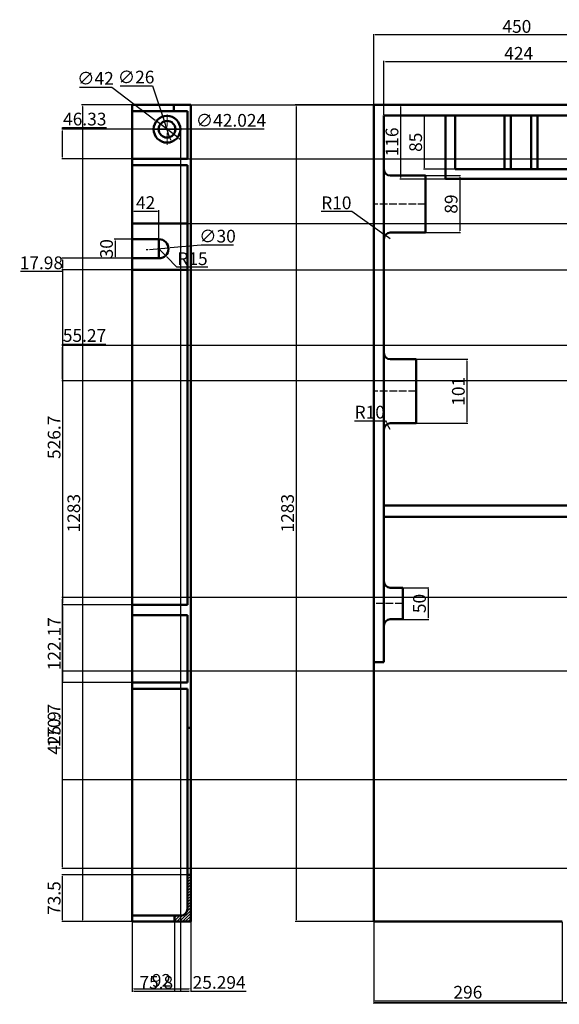
# Model space of a CAD drawing. Units: millimetres. Extents: x 1408 to 3734, y 1022 to 2569.
# Tile 1 of 3: x 1408 to 2256, y 1022 to 2569. Entities that reach past the tile are written whole.
import ezdxf

# ---------------------------------------------------------------- set-up
doc = ezdxf.new("R2010")
doc.units = ezdxf.units.MM
doc.linetypes.add('ACAD_ISO02W100', pattern=[15, 12, -3])
doc.linetypes.add('CENTER2', pattern=[28.575, 19.05, -3.175, 3.175, -3.175])
for name, color, linetype, lineweight in [('M-CNTR', 1, 'CENTER2', 18), ('M-DIMS', 2, 'Continuous', 25), ('M-HATC', 8, 'Continuous', 18), ('M-HIDN', 4, 'ACAD_ISO02W100', 25), ('M-OUTL', 7, 'Continuous', 50)]:
    doc.layers.add(name, color=color, linetype=linetype, lineweight=lineweight)
doc.styles.get("Standard").update_dxf_attribs({"font": 'arial.ttf'})
doc.dimstyles.new('ISO-25', dxfattribs={"dimtxt": 20, "dimasz": 2.5, "dimexe": 1.25, "dimexo": 0.625, "dimtad": 1, "dimtoh": 1, "dimdec": 0, "dimtxsty": 'Standard', "dimcen": 2.5, "dimadec": 0, "dimazin": 0, "dimtfac": 1, "dimtdec": 0, "dimtmove": 0, "dimatfit": 3, "dimfxl": 1, "dimarcsym": 0})

# ---------------------------------------------------------------- blocks, each defined once
blk = doc.blocks.new('*U3')
at = {"layer": 'M-CNTR', "color": 0, "transparency": 16777216}
for p, q in [((0, 4.2), (0, 24.5)), ((-24.5, 0), (-4.2, 0)), ((4.2, 0), (24.5, 0)), ((0, -24.5), (0, -4.2))]:
    blk.add_line(p, q, dxfattribs=at)
at = {"layer": 'M-CNTR', "color": 0, "linetype": 'Continuous', "transparency": 16777216}
for p, q in [((-2.1, 0), (2.1, 0)), ((0, -2.1), (0, 2.1))]:
    blk.add_line(p, q, dxfattribs=at)
blk = doc.blocks.new('*D4')
at = {"layer": 'Defpoints', "color": 0, "transparency": 16777216}
for p in [(1585, 2435.4), (1506.7, 1152.1), (1585, 1152.1)]:
    blk.add_point(p, dxfattribs=at)
at = {"layer": 'M-DIMS', "color": 0, "lineweight": -2, "transparency": 16777216}
for p, q in [((1584.3, 2435.4), (1505.4, 2435.4)), ((1506.7, 2432.9), (1506.7, 1154.6)), ((1584.3, 1152.1), (1505.4, 1152.1))]:
    blk.add_line(p, q, dxfattribs=at)
at = {"layer": 'M-DIMS', "color": 0, "transparency": 16777216}
for points in [[(1506.2, 2432.9), (1507.1, 2432.9), (1506.7, 2435.4)], [(1506.2, 1154.6), (1507.1, 1154.6), (1506.7, 1152.1)]]:
    blk.add_solid(points, dxfattribs=at)
at = {"layer": 'M-DIMS', "color": 0, "transparency": 16777216, "insert": (1495.8, 1793.7), "char_height": 20, "attachment_point": 5, "rotation": 90}
blk.add_mtext('1283', dxfattribs=at)
blk = doc.blocks.new('*D5')
at = {"layer": 'Defpoints', "color": 0, "transparency": 16777216}
for p in [(1585, 1152.1), (1677, 1152.1), (1677, 1046.1)]:
    blk.add_point(p, dxfattribs=at)
at = {"layer": 'M-DIMS', "color": 0, "lineweight": -2, "transparency": 16777216}
for p, q in [((1585, 1151.5), (1585, 1044.9)), ((1677, 1151.5), (1677, 1044.9)), ((1587.5, 1046.1), (1674.5, 1046.1))]:
    blk.add_line(p, q, dxfattribs=at)
at = {"layer": 'M-DIMS', "color": 0, "transparency": 16777216}
for points in [[(1587.5, 1046.5), (1587.5, 1045.7), (1585, 1046.1)], [(1674.5, 1046.5), (1674.5, 1045.7), (1677, 1046.1)]]:
    blk.add_solid(points, dxfattribs=at)
at = {"layer": 'M-DIMS', "color": 0, "transparency": 16777216, "insert": (1631, 1056.9), "char_height": 20, "attachment_point": 5}
blk.add_mtext('92', dxfattribs=at)
blk = doc.blocks.new('*D6')
at = {"layer": 'Defpoints', "color": 0, "transparency": 16777216}
for p in [(1964.7, 1152.1), (2260.7, 1152.1), (2260.7, 1027.5)]:
    blk.add_point(p, dxfattribs=at)
at = {"layer": 'M-DIMS', "color": 0, "lineweight": -2, "transparency": 16777216}
for p, q in [((1964.7, 1151.5), (1964.7, 1026.2)), ((2260.7, 1151.5), (2260.7, 1026.2)), ((1967.2, 1027.5), (2258.2, 1027.5))]:
    blk.add_line(p, q, dxfattribs=at)
at = {"layer": 'M-DIMS', "color": 0, "transparency": 16777216}
for points in [[(1967.2, 1027.9), (1967.2, 1027.1), (1964.7, 1027.5)], [(2258.2, 1027.9), (2258.2, 1027.1), (2260.7, 1027.5)]]:
    blk.add_solid(points, dxfattribs=at)
at = {"layer": 'M-DIMS', "color": 0, "transparency": 16777216, "insert": (2112.7, 1038.3), "char_height": 20, "attachment_point": 5}
blk.add_mtext('296', dxfattribs=at)
blk = doc.blocks.new('*D7')
at = {"layer": 'Defpoints', "color": 0, "transparency": 16777216}
for p in [(2814.7, 1219.4), (1964.7, 1152.1), (2814.7, 1025)]:
    blk.add_point(p, dxfattribs=at)
at = {"layer": 'M-DIMS', "color": 0, "lineweight": -2, "transparency": 16777216}
for p, q in [((2814.7, 1218.8), (2814.7, 1023.8)), ((1964.7, 1151.5), (1964.7, 1023.8)), ((1967.2, 1025), (2812.2, 1025))]:
    blk.add_line(p, q, dxfattribs=at)
at = {"layer": 'M-DIMS', "color": 0, "transparency": 16777216}
for points in [[(1967.2, 1025.5), (1967.2, 1024.6), (1964.7, 1025)], [(2812.2, 1025.5), (2812.2, 1024.6), (2814.7, 1025)]]:
    blk.add_solid(points, dxfattribs=at)
at = {"layer": 'M-DIMS', "color": 0, "transparency": 16777216, "insert": (2389.7, 1035.9), "char_height": 20, "attachment_point": 5}
blk.add_mtext('850', dxfattribs=at)
blk = doc.blocks.new('*D8')
at = {"layer": 'Defpoints', "color": 0, "transparency": 16777216}
for p in [(3556.7, 1373.9), (1964.7, 1152.1), (3556.7, 1024.2)]:
    blk.add_point(p, dxfattribs=at)
at = {"layer": 'M-DIMS', "color": 0, "lineweight": -2, "transparency": 16777216}
for p, q in [((3556.7, 1373.3), (3556.7, 1022.9)), ((1964.7, 1151.5), (1964.7, 1022.9)), ((1967.2, 1024.2), (3554.2, 1024.2))]:
    blk.add_line(p, q, dxfattribs=at)
at = {"layer": 'M-DIMS', "color": 0, "transparency": 16777216}
for points in [[(1967.2, 1024.6), (1967.2, 1023.8), (1964.7, 1024.2)], [(3554.2, 1024.6), (3554.2, 1023.8), (3556.7, 1024.2)]]:
    blk.add_solid(points, dxfattribs=at)
at = {"layer": 'M-DIMS', "color": 0, "transparency": 16777216, "insert": (2760.7, 1035), "char_height": 20, "attachment_point": 5}
blk.add_mtext('1592', dxfattribs=at)
blk = doc.blocks.new('*D9')
at = {"layer": 'Defpoints', "color": 0, "transparency": 16777216}
for p in [(1964.7, 2435.4), (1842.6, 1152.1), (1964.7, 1152.1)]:
    blk.add_point(p, dxfattribs=at)
at = {"layer": 'M-DIMS', "color": 0, "lineweight": -2, "transparency": 16777216}
for p, q in [((1964.1, 2435.4), (1841.4, 2435.4)), ((1842.6, 2432.9), (1842.6, 1154.6)), ((1964.1, 1152.1), (1841.4, 1152.1))]:
    blk.add_line(p, q, dxfattribs=at)
at = {"layer": 'M-DIMS', "color": 0, "transparency": 16777216}
for points in [[(1842.2, 2432.9), (1843, 2432.9), (1842.6, 2435.4)], [(1842.2, 1154.6), (1843, 1154.6), (1842.6, 1152.1)]]:
    blk.add_solid(points, dxfattribs=at)
at = {"layer": 'M-DIMS', "color": 0, "transparency": 16777216, "insert": (1831.8, 1793.7), "char_height": 20, "attachment_point": 5, "rotation": 90}
blk.add_mtext('1283', dxfattribs=at)
blk = doc.blocks.new('*D13')
at = {"layer": 'Defpoints', "color": 0, "transparency": 16777216}
for p in [(1964.7, 2545.3), (1964.7, 2435.4), (2414.7, 2435.4)]:
    blk.add_point(p, dxfattribs=at)
at = {"layer": 'M-DIMS', "color": 0, "lineweight": -2, "transparency": 16777216}
for p, q in [((1964.7, 2436), (1964.7, 2546.6)), ((2412.2, 2545.3), (1967.2, 2545.3)), ((2414.7, 2436), (2414.7, 2546.6))]:
    blk.add_line(p, q, dxfattribs=at)
at = {"layer": 'M-DIMS', "color": 0, "transparency": 16777216}
for points in [[(1967.2, 2545.7), (1967.2, 2544.9), (1964.7, 2545.3)], [(2412.2, 2545.7), (2412.2, 2544.9), (2414.7, 2545.3)]]:
    blk.add_solid(points, dxfattribs=at)
at = {"layer": 'M-DIMS', "color": 0, "transparency": 16777216, "insert": (2189.7, 2556.1), "char_height": 20, "attachment_point": 5}
blk.add_mtext('450', dxfattribs=at)
blk = doc.blocks.new('*D20')
at = {"layer": 'Defpoints', "color": 0, "transparency": 16777216}
for p in [(1623, 2409.8), (1656.5, 2384.4)]:
    blk.add_point(p, dxfattribs=at)
at = {"layer": 'M-DIMS', "color": 0, "lineweight": -2, "transparency": 16777216}
for p, q in [((1502.2, 2463.1), (1553, 2463.1)), ((1553, 2463.1), (1621, 2411.3)), ((1656.5, 2384.4), (1623, 2409.8)), ((1658.5, 2382.9), (1660.5, 2381.4))]:
    blk.add_line(p, q, dxfattribs=at)
at = {"layer": 'M-DIMS', "color": 0, "transparency": 16777216}
for points in [[(1621.3, 2411.7), (1620.8, 2411), (1623, 2409.8)], [(1658.7, 2383.2), (1658.2, 2382.6), (1656.5, 2384.4)]]:
    blk.add_solid(points, dxfattribs=at)
at = {"layer": 'M-DIMS', "color": 0, "transparency": 16777216, "insert": (1527.3, 2474.5), "char_height": 20, "attachment_point": 5}
blk.add_mtext('∅42', dxfattribs=at)
blk = doc.blocks.new('*D21')
at = {"layer": 'Defpoints', "color": 0, "transparency": 16777216}
for p in [(1635.6, 2409.5), (1643.9, 2384.7)]:
    blk.add_point(p, dxfattribs=at)
at = {"layer": 'M-DIMS', "color": 0, "lineweight": -2, "transparency": 16777216}
for p, q in [((1566, 2465.1), (1617, 2465.1)), ((1617, 2465.1), (1634.8, 2411.9)), ((1643.9, 2384.7), (1635.6, 2409.5)), ((1644.7, 2382.3), (1645.5, 2379.9))]:
    blk.add_line(p, q, dxfattribs=at)
at = {"layer": 'M-DIMS', "color": 0, "transparency": 16777216}
for points in [[(1635.2, 2412), (1634.4, 2411.8), (1635.6, 2409.5)], [(1645.1, 2382.4), (1644.3, 2382.2), (1643.9, 2384.7)]]:
    blk.add_solid(points, dxfattribs=at)
at = {"layer": 'M-DIMS', "color": 0, "transparency": 16777216, "insert": (1591.2, 2476.5), "char_height": 20, "attachment_point": 5}
blk.add_mtext('∅26', dxfattribs=at)
blk = doc.blocks.new('*D22')
at = {"layer": 'Defpoints', "color": 0, "transparency": 16777216}
for p in [(1612.2, 2208), (1642.1, 2210.6)]:
    blk.add_point(p, dxfattribs=at)
at = {"layer": 'M-DIMS', "color": 0, "lineweight": -2, "transparency": 16777216}
for p, q in [((1693.4, 2215.1), (1644.6, 2210.8)), ((1744.3, 2215.1), (1693.4, 2215.1)), ((1609.7, 2207.7), (1607.2, 2207.5)), ((1612.2, 2208), (1642.1, 2210.6))]:
    blk.add_line(p, q, dxfattribs=at)
at = {"layer": 'M-DIMS', "color": 0, "transparency": 16777216}
for points in [[(1609.7, 2208.1), (1609.7, 2207.3), (1612.2, 2208)], [(1644.5, 2211.2), (1644.6, 2210.4), (1642.1, 2210.6)]]:
    blk.add_solid(points, dxfattribs=at)
at = {"layer": 'M-DIMS', "color": 0, "transparency": 16777216, "insert": (1719.1, 2226.5), "char_height": 20, "attachment_point": 5}
blk.add_mtext('∅30', dxfattribs=at)
blk = doc.blocks.new('*D23')
at = {"layer": 'Defpoints', "color": 0, "transparency": 16777216}
for p in [(1627.1, 2268.5), (1585, 2224.3), (1627.1, 2224.3)]:
    blk.add_point(p, dxfattribs=at)
at = {"layer": 'M-DIMS', "color": 0, "lineweight": -2, "transparency": 16777216}
for p, q in [((1585, 2224.9), (1585, 2269.8)), ((1587.5, 2268.5), (1624.6, 2268.5)), ((1627.1, 2224.9), (1627.1, 2269.8))]:
    blk.add_line(p, q, dxfattribs=at)
at = {"layer": 'M-DIMS', "color": 0, "transparency": 16777216}
for points in [[(1587.5, 2268.9), (1587.5, 2268.1), (1585, 2268.5)], [(1624.6, 2268.9), (1624.6, 2268.1), (1627.1, 2268.5)]]:
    blk.add_solid(points, dxfattribs=at)
at = {"layer": 'M-DIMS', "color": 0, "transparency": 16777216, "insert": (1606.1, 2279.2), "char_height": 20, "attachment_point": 5}
blk.add_mtext('42', dxfattribs=at)
blk = doc.blocks.new('*D24')
at = {"layer": 'Defpoints', "color": 0, "transparency": 16777216}
for p in [(1585, 2224.3), (1558.1, 2194.3), (1585, 2194.3)]:
    blk.add_point(p, dxfattribs=at)
at = {"layer": 'M-DIMS', "color": 0, "lineweight": -2, "transparency": 16777216}
for p, q in [((1584.3, 2224.3), (1556.9, 2224.3)), ((1558.1, 2221.8), (1558.1, 2196.8)), ((1584.3, 2194.3), (1556.9, 2194.3))]:
    blk.add_line(p, q, dxfattribs=at)
at = {"layer": 'M-DIMS', "color": 0, "transparency": 16777216}
for points in [[(1557.7, 2221.8), (1558.6, 2221.8), (1558.1, 2224.3)], [(1557.7, 2196.8), (1558.6, 2196.8), (1558.1, 2194.3)]]:
    blk.add_solid(points, dxfattribs=at)
at = {"layer": 'M-DIMS', "color": 0, "transparency": 16777216, "insert": (1547.3, 2209.3), "char_height": 20, "attachment_point": 5, "rotation": 90}
blk.add_mtext('30', dxfattribs=at)
blk = doc.blocks.new('*D30')
at = {"layer": 'Defpoints', "color": 0, "transparency": 16777216}
for p in [(2031.3, 2035.6), (2031.3, 1935), (2111.2, 1935)]:
    blk.add_point(p, dxfattribs=at)
at = {"layer": 'M-DIMS', "color": 0, "lineweight": -2, "transparency": 16777216}
for p, q in [((2031.9, 2035.6), (2112.4, 2035.6)), ((2111.2, 2033.1), (2111.2, 1937.5)), ((2031.9, 1935), (2112.4, 1935))]:
    blk.add_line(p, q, dxfattribs=at)
at = {"layer": 'M-DIMS', "color": 0, "transparency": 16777216}
for points in [[(2110.8, 2033.1), (2111.6, 2033.1), (2111.2, 2035.6)], [(2110.8, 1937.5), (2111.6, 1937.5), (2111.2, 1935)]]:
    blk.add_solid(points, dxfattribs=at)
at = {"layer": 'M-DIMS', "color": 0, "transparency": 16777216, "insert": (2100.3, 1985.3), "char_height": 20, "attachment_point": 5, "rotation": 90}
blk.add_mtext('101', dxfattribs=at)
blk = doc.blocks.new('*D31')
at = {"layer": 'Defpoints', "color": 0, "transparency": 16777216}
for p in [(2010.5, 1676.6), (2010.5, 1626.9), (2050.1, 1626.9)]:
    blk.add_point(p, dxfattribs=at)
at = {"layer": 'M-DIMS', "color": 0, "lineweight": -2, "transparency": 16777216}
for p, q in [((2011.1, 1676.6), (2051.3, 1676.6)), ((2050.1, 1674.1), (2050.1, 1629.4)), ((2011.1, 1626.9), (2051.3, 1626.9))]:
    blk.add_line(p, q, dxfattribs=at)
at = {"layer": 'M-DIMS', "color": 0, "transparency": 16777216}
for points in [[(2049.6, 1674.1), (2050.5, 1674.1), (2050.1, 1676.6)], [(2049.6, 1629.4), (2050.5, 1629.4), (2050.1, 1626.9)]]:
    blk.add_solid(points, dxfattribs=at)
at = {"layer": 'M-DIMS', "color": 0, "transparency": 16777216, "insert": (2039.2, 1651.8), "char_height": 20, "attachment_point": 5, "rotation": 90}
blk.add_mtext('50', dxfattribs=at)
blk = doc.blocks.new('*D32')
at = {"layer": 'Defpoints', "color": 0, "transparency": 16777216}
for p in [(2046.2, 2324.2), (2046.2, 2234.8), (2099.8, 2234.8)]:
    blk.add_point(p, dxfattribs=at)
at = {"layer": 'M-DIMS', "color": 0, "lineweight": -2, "transparency": 16777216}
for p, q in [((2046.8, 2324.2), (2101.1, 2324.2)), ((2099.8, 2321.7), (2099.8, 2237.3)), ((2046.8, 2234.8), (2101.1, 2234.8))]:
    blk.add_line(p, q, dxfattribs=at)
at = {"layer": 'M-DIMS', "color": 0, "transparency": 16777216}
for points in [[(2099.4, 2321.7), (2100.2, 2321.7), (2099.8, 2324.2)], [(2099.4, 2237.3), (2100.2, 2237.3), (2099.8, 2234.8)]]:
    blk.add_solid(points, dxfattribs=at)
at = {"layer": 'M-DIMS', "color": 0, "transparency": 16777216, "insert": (2089, 2279.5), "char_height": 20, "attachment_point": 5, "rotation": 90}
blk.add_mtext('89', dxfattribs=at)
blk = doc.blocks.new('*D33')
at = {"layer": 'Defpoints', "color": 0, "transparency": 16777216}
for p in [(1982.5, 2230.7), (1990.7, 2224.8)]:
    blk.add_point(p, dxfattribs=at)
at = {"layer": 'M-DIMS', "color": 0, "lineweight": -2, "transparency": 16777216}
for p, q in [((1882, 2268.1), (1930.4, 2268.1)), ((1930.4, 2268.1), (1980.5, 2232.1)), ((1990.7, 2224.8), (1982.5, 2230.7))]:
    blk.add_line(p, q, dxfattribs=at)
at = {"layer": 'M-DIMS', "color": 0, "transparency": 16777216}
blk.add_solid([(1980.7, 2232.4), (1980.3, 2231.8), (1982.5, 2230.7)], dxfattribs=at)
at = {"layer": 'M-DIMS', "color": 0, "transparency": 16777216, "insert": (1905.9, 2278.9), "char_height": 20, "attachment_point": 5}
blk.add_mtext('R10', dxfattribs=at)
blk = doc.blocks.new('*D34')
at = {"layer": 'Defpoints', "color": 0, "transparency": 16777216}
for p in [(1980.7, 2503.2), (1980.7, 2418.9), (2404.5, 2417.1)]:
    blk.add_point(p, dxfattribs=at)
at = {"layer": 'M-DIMS', "color": 0, "lineweight": -2, "transparency": 16777216}
for p, q in [((1980.7, 2419.6), (1980.7, 2504.4)), ((2402, 2503.2), (1983.2, 2503.2)), ((2404.5, 2417.7), (2404.5, 2504.4))]:
    blk.add_line(p, q, dxfattribs=at)
at = {"layer": 'M-DIMS', "color": 0, "transparency": 16777216}
for points in [[(1983.2, 2503.6), (1983.2, 2502.8), (1980.7, 2503.2)], [(2402, 2503.6), (2402, 2502.8), (2404.5, 2503.2)]]:
    blk.add_solid(points, dxfattribs=at)
at = {"layer": 'M-DIMS', "color": 0, "transparency": 16777216, "insert": (2192.6, 2513.8), "char_height": 20, "attachment_point": 5}
blk.add_mtext('424', dxfattribs=at)
blk = doc.blocks.new('*D35')
at = {"layer": 'Defpoints', "color": 0, "transparency": 16777216}
for p in [(2190.9, 2418.9), (2044, 2334.2), (2252.1, 2334.2)]:
    blk.add_point(p, dxfattribs=at)
at = {"layer": 'M-DIMS', "color": 0, "lineweight": -2, "transparency": 16777216}
for p, q in [((2190.3, 2418.9), (2042.8, 2418.9)), ((2044, 2416.4), (2044, 2336.7)), ((2251.5, 2334.2), (2042.8, 2334.2))]:
    blk.add_line(p, q, dxfattribs=at)
at = {"layer": 'M-DIMS', "color": 0, "transparency": 16777216}
for points in [[(2043.6, 2416.4), (2044.4, 2416.4), (2044, 2418.9)], [(2043.6, 2336.7), (2044.4, 2336.7), (2044, 2334.2)]]:
    blk.add_solid(points, dxfattribs=at)
at = {"layer": 'M-DIMS', "color": 0, "transparency": 16777216, "insert": (2033.2, 2376.6), "char_height": 20, "attachment_point": 5, "rotation": 90}
blk.add_mtext('85', dxfattribs=at)
blk = doc.blocks.new('*D36')
at = {"layer": 'Defpoints', "color": 0, "transparency": 16777216}
for p in [(2189.7, 2435.4), (2006.9, 2318.9), (2231.1, 2318.9)]:
    blk.add_point(p, dxfattribs=at)
at = {"layer": 'M-DIMS', "color": 0, "lineweight": -2, "transparency": 16777216}
for p, q in [((2189.1, 2435.4), (2005.6, 2435.4)), ((2006.9, 2432.9), (2006.9, 2321.4)), ((2230.5, 2318.9), (2005.6, 2318.9))]:
    blk.add_line(p, q, dxfattribs=at)
at = {"layer": 'M-DIMS', "color": 0, "transparency": 16777216}
for points in [[(2006.5, 2432.9), (2007.3, 2432.9), (2006.9, 2435.4)], [(2006.5, 2321.4), (2007.3, 2321.4), (2006.9, 2318.9)]]:
    blk.add_solid(points, dxfattribs=at)
at = {"layer": 'M-DIMS', "color": 0, "transparency": 16777216, "insert": (1996, 2377.2), "char_height": 20, "attachment_point": 5, "rotation": 90}
blk.add_mtext('116', dxfattribs=at)
blk = doc.blocks.new('*D40')
at = {"layer": 'Defpoints', "color": 0, "transparency": 16777216}
for p in [(1660.8, 2397.1), (1585, 2350.8), (1660.8, 1042.8)]:
    blk.add_point(p, dxfattribs=at)
at = {"layer": 'M-DIMS', "color": 0, "lineweight": -2, "transparency": 16777216}
for p, q in [((1660.8, 2396.5), (1660.8, 1041.6)), ((1585, 2350.2), (1585, 1041.6)), ((1587.5, 1042.8), (1658.3, 1042.8))]:
    blk.add_line(p, q, dxfattribs=at)
at = {"layer": 'M-DIMS', "color": 0, "transparency": 16777216}
for points in [[(1587.5, 1043.3), (1587.5, 1042.4), (1585, 1042.8)], [(1658.3, 1043.3), (1658.3, 1042.4), (1660.8, 1042.8)]]:
    blk.add_solid(points, dxfattribs=at)
at = {"layer": 'M-DIMS', "color": 0, "transparency": 16777216, "insert": (1622.9, 1053.7), "char_height": 20, "attachment_point": 5}
blk.add_mtext('75.8', dxfattribs=at)
blk = doc.blocks.new('*D41')
at = {"layer": 'Defpoints', "color": 0, "transparency": 16777216}
for p in [(1475.7, 2397.1), (1660.8, 2397.1), (1585, 2350.8)]:
    blk.add_point(p, dxfattribs=at)
at = {"layer": 'M-DIMS', "color": 0, "lineweight": -2, "transparency": 16777216}
for p, q in [((1475.7, 2397.1), (1475.7, 2399.6)), ((1475.7, 2399.6), (1544.6, 2399.6)), ((1660.1, 2397.1), (1474.5, 2397.1)), ((1475.7, 2353.3), (1475.7, 2394.6)), ((1584.3, 2350.8), (1474.5, 2350.8))]:
    blk.add_line(p, q, dxfattribs=at)
at = {"layer": 'M-DIMS', "color": 0, "transparency": 16777216}
for points in [[(1475.3, 2394.6), (1476.1, 2394.6), (1475.7, 2397.1)], [(1475.3, 2353.3), (1476.1, 2353.3), (1475.7, 2350.8)]]:
    blk.add_solid(points, dxfattribs=at)
at = {"layer": 'M-DIMS', "color": 0, "transparency": 16777216, "insert": (1510.5, 2410.5), "char_height": 20, "attachment_point": 5}
blk.add_mtext('46.33', dxfattribs=at)
blk = doc.blocks.new('*D42')
at = {"layer": 'Defpoints', "color": 0, "transparency": 16777216}
for p in [(1677, 2435.4), (1671.8, 2350.8), (3665.9, 2350.8)]:
    blk.add_point(p, dxfattribs=at)
at = {"layer": 'M-DIMS', "color": 0, "lineweight": -2, "transparency": 16777216}
for p, q in [((1677.6, 2435.4), (3667.2, 2435.4)), ((3665.9, 2432.9), (3665.9, 2353.3)), ((1672.5, 2350.8), (3667.2, 2350.8))]:
    blk.add_line(p, q, dxfattribs=at)
at = {"layer": 'M-DIMS', "color": 0, "transparency": 16777216}
for points in [[(3665.5, 2432.9), (3666.4, 2432.9), (3665.9, 2435.4)], [(3665.5, 2353.3), (3666.4, 2353.3), (3665.9, 2350.8)]]:
    blk.add_solid(points, dxfattribs=at)
at = {"layer": 'M-DIMS', "color": 0, "transparency": 16777216, "insert": (3655.1, 2393.1), "char_height": 20, "attachment_point": 5, "rotation": 90}
blk.add_mtext('84.6', dxfattribs=at)
blk = doc.blocks.new('*D43')
at = {"layer": 'Defpoints', "color": 0, "transparency": 16777216}
for p in [(1671.8, 2350.8), (1671.8, 2249.2), (3665.9, 2249.2)]:
    blk.add_point(p, dxfattribs=at)
at = {"layer": 'M-DIMS', "color": 0, "lineweight": -2, "transparency": 16777216}
for p, q in [((1672.5, 2350.8), (3667.2, 2350.8)), ((3665.9, 2348.3), (3665.9, 2251.7)), ((1672.5, 2249.2), (3667.2, 2249.2))]:
    blk.add_line(p, q, dxfattribs=at)
at = {"layer": 'M-DIMS', "color": 0, "transparency": 16777216}
for points in [[(3665.5, 2348.3), (3666.4, 2348.3), (3665.9, 2350.8)], [(3665.5, 2251.7), (3666.4, 2251.7), (3665.9, 2249.2)]]:
    blk.add_solid(points, dxfattribs=at)
at = {"layer": 'M-DIMS', "color": 0, "transparency": 16777216, "insert": (3655.1, 2300), "char_height": 20, "attachment_point": 5, "rotation": 90}
blk.add_mtext('101.6', dxfattribs=at)
blk = doc.blocks.new('*D44')
at = {"layer": 'Defpoints', "color": 0, "transparency": 16777216}
for p in [(1671.8, 2249.2), (1671.8, 2176.3), (3665.9, 2176.3)]:
    blk.add_point(p, dxfattribs=at)
at = {"layer": 'M-DIMS', "color": 0, "lineweight": -2, "transparency": 16777216}
for p, q in [((1672.5, 2249.2), (3667.2, 2249.2)), ((3665.9, 2246.7), (3665.9, 2178.8)), ((1672.5, 2176.3), (3667.2, 2176.3))]:
    blk.add_line(p, q, dxfattribs=at)
at = {"layer": 'M-DIMS', "color": 0, "transparency": 16777216}
for points in [[(3665.5, 2246.7), (3666.4, 2246.7), (3665.9, 2249.2)], [(3665.5, 2178.8), (3666.4, 2178.8), (3665.9, 2176.3)]]:
    blk.add_solid(points, dxfattribs=at)
at = {"layer": 'M-DIMS', "color": 0, "transparency": 16777216, "insert": (3655.1, 2212.7), "char_height": 20, "attachment_point": 5, "rotation": 90}
blk.add_mtext('72.9', dxfattribs=at)
blk = doc.blocks.new('*D45')
at = {"layer": 'Defpoints', "color": 0, "transparency": 16777216}
for p in [(1671.8, 2176.3), (1475.7, 1649.6), (1671.8, 1649.6)]:
    blk.add_point(p, dxfattribs=at)
at = {"layer": 'M-DIMS', "color": 0, "lineweight": -2, "transparency": 16777216}
for p, q in [((1671.2, 2176.3), (1474.5, 2176.3)), ((1475.7, 2173.8), (1475.7, 1652.1)), ((1671.2, 1649.6), (1474.5, 1649.6))]:
    blk.add_line(p, q, dxfattribs=at)
at = {"layer": 'M-DIMS', "color": 0, "transparency": 16777216}
for points in [[(1475.3, 2173.8), (1476.1, 2173.8), (1475.7, 2176.3)], [(1475.3, 1652.1), (1476.1, 1652.1), (1475.7, 1649.6)]]:
    blk.add_solid(points, dxfattribs=at)
at = {"layer": 'M-DIMS', "color": 0, "transparency": 16777216, "insert": (1464.9, 1912.9), "char_height": 20, "attachment_point": 5, "rotation": 90}
blk.add_mtext('526.7', dxfattribs=at)
blk = doc.blocks.new('*D46')
at = {"layer": 'Defpoints', "color": 0, "transparency": 16777216}
for p in [(1671.8, 1649.6), (1475.7, 1527.4), (1671.8, 1527.4)]:
    blk.add_point(p, dxfattribs=at)
at = {"layer": 'M-DIMS', "color": 0, "lineweight": -2, "transparency": 16777216}
for p, q in [((1671.2, 1649.6), (1474.5, 1649.6)), ((1475.7, 1647.1), (1475.7, 1529.9)), ((1671.2, 1527.4), (1474.5, 1527.4))]:
    blk.add_line(p, q, dxfattribs=at)
at = {"layer": 'M-DIMS', "color": 0, "transparency": 16777216}
for points in [[(1475.3, 1647.1), (1476.1, 1647.1), (1475.7, 1649.6)], [(1475.3, 1529.9), (1476.1, 1529.9), (1475.7, 1527.4)]]:
    blk.add_solid(points, dxfattribs=at)
at = {"layer": 'M-DIMS', "color": 0, "transparency": 16777216, "insert": (1465, 1588.5), "char_height": 20, "attachment_point": 5, "rotation": 90}
blk.add_mtext('122.17', dxfattribs=at)
blk = doc.blocks.new('*D47')
at = {"layer": 'Defpoints', "color": 0, "transparency": 16777216}
for p in [(1585, 2194.3), (1475.7, 2176.3), (1585, 2176.3)]:
    blk.add_point(p, dxfattribs=at)
at = {"layer": 'M-DIMS', "color": 0, "lineweight": -2, "transparency": 16777216}
for p, q in [((1584.3, 2194.3), (1474.5, 2194.3)), ((1475.7, 2191.8), (1475.7, 2178.8)), ((1475.7, 2173.8), (1409.4, 2173.8)), ((1584.3, 2176.3), (1474.5, 2176.3)), ((1475.7, 2176.3), (1475.7, 2173.8))]:
    blk.add_line(p, q, dxfattribs=at)
at = {"layer": 'M-DIMS', "color": 0, "transparency": 16777216}
for points in [[(1475.3, 2191.8), (1476.1, 2191.8), (1475.7, 2194.3)], [(1475.3, 2178.8), (1476.1, 2178.8), (1475.7, 2176.3)]]:
    blk.add_solid(points, dxfattribs=at)
at = {"layer": 'M-DIMS', "color": 0, "transparency": 16777216, "insert": (1442.3, 2184.6), "char_height": 20, "attachment_point": 5}
blk.add_mtext('17.98', dxfattribs=at)
blk = doc.blocks.new('*D48')
at = {"layer": 'Defpoints', "color": 0, "transparency": 16777216}
for p in [(1475.7, 1225.6), (1677, 1225.6), (1677, 1152.1)]:
    blk.add_point(p, dxfattribs=at)
at = {"layer": 'M-DIMS', "color": 0, "lineweight": -2, "transparency": 16777216}
for p, q in [((1676.3, 1225.6), (1474.5, 1225.6)), ((1475.7, 1154.6), (1475.7, 1223.1)), ((1676.3, 1152.1), (1474.5, 1152.1))]:
    blk.add_line(p, q, dxfattribs=at)
at = {"layer": 'M-DIMS', "color": 0, "transparency": 16777216}
for points in [[(1475.3, 1223.1), (1476.1, 1223.1), (1475.7, 1225.6)], [(1475.3, 1154.6), (1476.1, 1154.6), (1475.7, 1152.1)]]:
    blk.add_solid(points, dxfattribs=at)
at = {"layer": 'M-DIMS', "color": 0, "transparency": 16777216, "insert": (1464.9, 1188.8), "char_height": 20, "attachment_point": 5, "rotation": 90}
blk.add_mtext('73.5', dxfattribs=at)
blk = doc.blocks.new('*D49')
at = {"layer": 'Defpoints', "color": 0, "transparency": 16777216}
for p in [(1651.7, 1152.1), (1677, 1152.1), (1677, 1042.8)]:
    blk.add_point(p, dxfattribs=at)
at = {"layer": 'M-DIMS', "color": 0, "lineweight": -2, "transparency": 16777216}
for p, q in [((1651.7, 1151.5), (1651.7, 1041.6)), ((1677, 1151.5), (1677, 1041.6)), ((1654.2, 1042.8), (1674.5, 1042.8)), ((1677, 1042.8), (1764, 1042.8))]:
    blk.add_line(p, q, dxfattribs=at)
at = {"layer": 'M-DIMS', "color": 0, "transparency": 16777216}
for points in [[(1654.2, 1043.3), (1654.2, 1042.4), (1651.7, 1042.8)], [(1674.5, 1043.3), (1674.5, 1042.4), (1677, 1042.8)]]:
    blk.add_solid(points, dxfattribs=at)
at = {"layer": 'M-DIMS', "color": 0, "transparency": 16777216, "insert": (1721.7, 1053.7), "char_height": 20, "attachment_point": 5}
blk.add_mtext('25.294', dxfattribs=at)
blk = doc.blocks.new('*D50')
at = {"layer": 'Defpoints', "color": 0, "transparency": 16777216}
for p in [(1475.7, 2057.1), (3047.3, 2057.1), (3014.5, 2001.8)]:
    blk.add_point(p, dxfattribs=at)
at = {"layer": 'M-DIMS', "color": 0, "lineweight": -2, "transparency": 16777216}
for p, q in [((1475.7, 2057.1), (1475.7, 2059.6)), ((1475.7, 2059.6), (1543.8, 2059.6)), ((3046.6, 2057.1), (1474.5, 2057.1)), ((1475.7, 2004.3), (1475.7, 2054.6)), ((3013.9, 2001.8), (1474.5, 2001.8))]:
    blk.add_line(p, q, dxfattribs=at)
at = {"layer": 'M-DIMS', "color": 0, "transparency": 16777216}
for points in [[(1475.3, 2054.6), (1476.1, 2054.6), (1475.7, 2057.1)], [(1475.3, 2004.3), (1476.1, 2004.3), (1475.7, 2001.8)]]:
    blk.add_solid(points, dxfattribs=at)
at = {"layer": 'M-DIMS', "color": 0, "transparency": 16777216, "insert": (1510.1, 2070.4), "char_height": 20, "attachment_point": 5}
blk.add_mtext('55.27', dxfattribs=at)
blk = doc.blocks.new('*D60')
at = {"layer": 'Defpoints', "color": 0, "transparency": 16777216}
for p in [(1475.7, 1661.3), (2298.6, 1661.3), (2298.6, 1235.4)]:
    blk.add_point(p, dxfattribs=at)
at = {"layer": 'M-DIMS', "color": 0, "lineweight": -2, "transparency": 16777216}
for p, q in [((2298, 1661.3), (1474.5, 1661.3)), ((1475.7, 1237.9), (1475.7, 1658.8)), ((2298, 1235.4), (1474.5, 1235.4))]:
    blk.add_line(p, q, dxfattribs=at)
at = {"layer": 'M-DIMS', "color": 0, "transparency": 16777216}
for points in [[(1475.3, 1658.8), (1476.1, 1658.8), (1475.7, 1661.3)], [(1475.3, 1237.9), (1476.1, 1237.9), (1475.7, 1235.4)]]:
    blk.add_solid(points, dxfattribs=at)
at = {"layer": 'M-DIMS', "color": 0, "transparency": 16777216, "insert": (1464.9, 1448.3), "char_height": 20, "attachment_point": 5, "rotation": 90}
blk.add_mtext('425.9', dxfattribs=at)
blk = doc.blocks.new('*D62')
at = {"layer": 'Defpoints', "color": 0, "transparency": 16777216}
for p in [(1475.7, 1545.3), (2452.5, 1545.3), (2379.1, 1374.6)]:
    blk.add_point(p, dxfattribs=at)
at = {"layer": 'M-DIMS', "color": 0, "lineweight": -2, "transparency": 16777216}
for p, q in [((2451.8, 1545.3), (1474.5, 1545.3)), ((1475.7, 1377.1), (1475.7, 1542.8)), ((2378.5, 1374.6), (1474.5, 1374.6))]:
    blk.add_line(p, q, dxfattribs=at)
at = {"layer": 'M-DIMS', "color": 0, "transparency": 16777216}
for points in [[(1475.3, 1542.8), (1476.1, 1542.8), (1475.7, 1545.3)], [(1475.3, 1377.1), (1476.1, 1377.1), (1475.7, 1374.6)]]:
    blk.add_solid(points, dxfattribs=at)
at = {"layer": 'M-DIMS', "color": 0, "transparency": 16777216, "insert": (1464.9, 1459.9), "char_height": 20, "attachment_point": 5, "rotation": 90}
blk.add_mtext('170.7', dxfattribs=at)
blk = doc.blocks.new('*D85')
at = {"layer": 'Defpoints', "color": 0, "transparency": 16777216}
for p in [(1618.7, 2397.1), (1660.8, 2397.1)]:
    blk.add_point(p, dxfattribs=at)
at = {"layer": 'M-DIMS', "color": 0, "lineweight": -2, "transparency": 16777216}
for p, q in [((1616.2, 2397.1), (1613.7, 2397.1)), ((1618.7, 2397.1), (1660.8, 2397.1)), ((1687.3, 2397.1), (1663.3, 2397.1)), ((1792.6, 2397.1), (1687.3, 2397.1))]:
    blk.add_line(p, q, dxfattribs=at)
at = {"layer": 'M-DIMS', "color": 0, "transparency": 16777216}
for points in [[(1616.2, 2397.5), (1616.2, 2396.7), (1618.7, 2397.1)], [(1663.3, 2397.5), (1663.3, 2396.7), (1660.8, 2397.1)]]:
    blk.add_solid(points, dxfattribs=at)
at = {"layer": 'M-DIMS', "color": 0, "transparency": 16777216, "insert": (1740.3, 2408.5), "char_height": 20, "attachment_point": 5}
blk.add_mtext('∅42.024', dxfattribs=at)
blk = doc.blocks.new('*D86')
at = {"layer": 'Defpoints', "color": 0, "transparency": 16777216}
for p in [(1627.1, 2209.3), (1637.5, 2198.5)]:
    blk.add_point(p, dxfattribs=at)
at = {"layer": 'M-DIMS', "color": 0, "lineweight": -2, "transparency": 16777216}
for p, q in [((1627.1, 2209.3), (1637.5, 2198.5)), ((1655.2, 2180.1), (1639.3, 2196.7)), ((1703.7, 2180.1), (1655.2, 2180.1))]:
    blk.add_line(p, q, dxfattribs=at)
at = {"layer": 'M-DIMS', "color": 0, "transparency": 16777216}
blk.add_solid([(1639.6, 2196.9), (1639, 2196.4), (1637.5, 2198.5)], dxfattribs=at)
at = {"layer": 'M-DIMS', "color": 0, "transparency": 16777216, "insert": (1679.8, 2191), "char_height": 20, "attachment_point": 5}
blk.add_mtext('R15', dxfattribs=at)
blk = doc.blocks.new('*D87')
at = {"layer": 'Defpoints', "color": 0, "transparency": 16777216}
for p in [(1985.8, 1933.8), (1990.7, 1925)]:
    blk.add_point(p, dxfattribs=at)
at = {"layer": 'M-DIMS', "color": 0, "lineweight": -2, "transparency": 16777216}
for p, q in [((1934.6, 1939.1), (1983, 1939.1)), ((1983, 1939.1), (1984.6, 1936)), ((1990.7, 1925), (1985.8, 1933.8))]:
    blk.add_line(p, q, dxfattribs=at)
at = {"layer": 'M-DIMS', "color": 0, "transparency": 16777216}
blk.add_solid([(1985, 1936.2), (1984.3, 1935.8), (1985.8, 1933.8)], dxfattribs=at)
at = {"layer": 'M-DIMS', "color": 0, "transparency": 16777216, "insert": (1958.5, 1949.9), "char_height": 20, "attachment_point": 5}
blk.add_mtext('R10', dxfattribs=at)

msp = doc.modelspace()

# ---------------------------------------------------------------- hatches: boundary and pattern name
at = {"layer": 'M-HATC'}
h = msp.add_hatch(dxfattribs=at)
h.set_pattern_fill('ANSI31', color=256)
h.paths.add_polyline_path([(1676.9655, 1219.3757), (1676.9655, 1225.5822), (1671.843, 1225.5822), (1671.843, 1219.3757), (1671.843, 1171.4252, -0.414213562), (1661.843, 1161.4252), (1651.6714, 1161.4252), (1651.6714, 1152.0867), (1676.9655, 1152.0867)])

# ---------------------------------------------------------------- linework, layer by layer
at = {"layer": 'M-HIDN'}
for p, q in [((2046.202, 2279.513), (1964.6991, 2279.513)), ((2031.2921, 1985.3002), (1964.6991, 1985.3002)), ((2010.4639, 1651.7582), (1964.6991, 1651.7582))]:
    msp.add_line(p, q, dxfattribs=at)
at = {"layer": 'M-OUTL'}
for p, q in [((1676.9655, 2435.3757), (1584.9655, 2435.3757)), ((1584.9655, 2435.3757), (1584.9655, 1152.0867)), ((1650.3694, 2425.5407), (1650.3694, 2435.3757)), ((1676.9655, 2435.3757), (1676.9655, 1219.3757)), ((1964.6991, 2435.3757), (1964.6991, 1219.3757)), ((1964.6991, 2435.3757), (2414.6991, 2435.3757)), ((1671.843, 2425.5407), (1584.9655, 2425.5407)), ((1671.843, 2425.5407), (1671.843, 2350.7788)), ((1980.6517, 2418.9311), (2401.1247, 2418.9311)), ((1980.6517, 2418.9311), (1980.6517, 2334.2036)), ((2077.4791, 2418.9311), (2077.4791, 2318.9311)), ((2092.8085, 2418.9311), (2092.8085, 2334.2032)), ((2170.0319, 2418.9311), (2170.0319, 2334.2032)), ((2180.0319, 2334.2032), (2180.0319, 2418.9311)), ((2212.0319, 2418.9311), (2212.0319, 2334.2032)), ((2222.0319, 2334.2032), (2222.0319, 2418.9311)), ((1584.9655, 2350.7788), (1671.843, 2350.7788)), ((1671.843, 2340.7788), (1584.9655, 2340.7788)), ((1671.843, 2340.7788), (1671.843, 1649.6019)), ((1980.6517, 2224.8225), (1980.6517, 2334.2036)), ((2046.202, 2324.2036), (1990.6517, 2324.2036)), ((2046.202, 2234.8225), (2046.202, 2324.2036)), ((2092.8085, 2334.2032), (2411.4791, 2334.2032)), ((2077.4791, 2318.9311), (2384.7504, 2318.9311)), ((1584.9655, 2249.1777), (1671.843, 2249.1777)), ((1990.6517, 2234.8225), (2046.202, 2234.8225)), ((1584.9655, 2224.2646), (1627.1403, 2224.2646)), ((1627.1403, 2224.2646), (1627.1403, 2194.2646)), ((1980.6517, 2224.8225), (1980.6517, 2045.5771)), ((1627.1403, 2194.2646), (1584.9655, 2194.2646)), ((1671.843, 2176.2838), (1584.9655, 2176.2838)), ((1980.6517, 1973.3926), (1980.6517, 2045.5771)), ((2031.2921, 2035.5771), (1990.6517, 2035.5771)), ((2031.2921, 1935.0233), (2031.2921, 2035.5771)), ((1980.6517, 1925.0233), (1980.6517, 1973.3926)), ((1990.6517, 1935.0233), (2031.2921, 1935.0233)), ((1980.6517, 1925.0233), (1980.6517, 1686.6065)), ((1980.6517, 1805.8149), (2798.6154, 1805.8149)), ((1980.6517, 1787.9634), (2798.6154, 1787.9634)), ((1980.6517, 1616.9099), (1980.6517, 1686.6065)), ((2010.4639, 1676.6065), (1990.6517, 1676.6065)), ((2010.4639, 1626.9099), (2010.4639, 1676.6065)), ((1584.9655, 1649.6019), (1671.843, 1649.6019)), ((1671.843, 1633.6019), (1584.9655, 1633.6019)), ((1671.843, 1633.6019), (1671.843, 1527.4292)), ((1990.6517, 1626.9099), (2010.4639, 1626.9099)), ((1980.6517, 1616.9099), (1980.6517, 1559.5606)), ((1964.6991, 1559.5606), (1980.6517, 1559.5606)), ((1584.9655, 1527.4292), (1671.843, 1527.4292)), ((1671.843, 1517.4292), (1584.9655, 1517.4292)), ((1671.843, 1517.4292), (1671.843, 1219.3757)), ((1671.843, 1456.2631), (1676.9655, 1456.2631)), ((1671.843, 1225.5822), (1676.9655, 1225.5822)), ((1671.843, 1219.3757), (1671.843, 1171.4252)), ((1676.9655, 1219.3757), (1676.9655, 1152.0867)), ((1964.6991, 1219.3757), (1964.6991, 1152.0867)), ((1661.843, 1161.4252), (1584.9655, 1161.4252)), ((1651.6714, 1161.4252), (1651.6714, 1152.0867)), ((1676.9655, 1152.0867), (1584.9655, 1152.0867)), ((1964.6991, 1152.0867), (2260.6991, 1152.0867))]:
    msp.add_line(p, q, dxfattribs=at)
for radius in [21.0121, 13.1116]:
    msp.add_circle((1639.7524, 2397.1126), radius, dxfattribs=at)
for centre, radius, start, end in [((1990.6517, 2334.2036), 10, 180, 270), ((1990.6517, 2224.8225), 10, 90, 180), ((1627.1403, 2209.2646), 15, 270, 90), ((1990.6517, 2045.5771), 10, 180, 270), ((1990.6517, 1925.0233), 10, 90, 180), ((1990.6517, 1686.6065), 10, 180, 270), ((1990.6517, 1616.9099), 10, 90, 180), ((1661.843, 1171.4252), 10, 270, 0)]:
    msp.add_arc(centre, radius, start, end, dxfattribs=at)

# ---------------------------------------------------------------- block references
at = {"layer": 'M-CNTR'}
msp.add_blockref('*U3', (1639.7524, 2397.1126), dxfattribs=at)

# ---------------------------------------------------------------- dimensions: what is measured, and where the dimension line sits
at = {"layer": 'M-DIMS'}
for base, p1, p2, override, picture, middle in [((1964.6991, 2545.3015), (2414.6991, 2435.3757), (1964.6991, 2435.3757), {"dimclrd": 0, "dimclre": 0, "dimclrt": 0}, '*D13', (2189.6991, 2556.138)), ((1980.6517, 2503.179), (2404.4571, 2417.0877), (1980.6517, 2418.9311), {"dimclrd": 0, "dimclre": 0, "dimclrt": 0}, '*D34', (2192.5544, 2513.8449)), ((1660.7645, 1042.8367), (1584.9655, 2350.7788), (1660.7645, 2397.1126), {"dimdec": 1, "dimlfac": 1, "dimrnd": 0, "dimzin": 0, "dimdsep": 46, "dimlunit": 2}, '*D40', (1622.865, 1053.6732)), ((1627.1403, 2268.5239), (1584.9655, 2224.2646), (1627.1403, 2224.2646), {"dimclrd": 0, "dimclre": 0, "dimclrt": 0}, '*D23', (1606.0529, 2279.1899)), ((3556.6991, 1024.195), (1964.6991, 1152.0867), (3556.6991, 1373.8764), {"dimclrd": 0, "dimclre": 0, "dimclrt": 0}, '*D8', (2760.6991, 1035.0315)), ((2814.6991, 1025.0488), (1964.6991, 1152.0867), (2814.6991, 1219.3757), {"dimclrd": 0, "dimclre": 0, "dimclrt": 0}, '*D7', (2389.6991, 1035.8853)), ((1676.9655, 1046.1076), (1584.9655, 1152.0867), (1676.9655, 1152.0867), {"dimclrd": 0, "dimclre": 0, "dimclrt": 0}, '*D5', (1630.9655, 1056.9441)), ((1676.9655, 1042.8367), (1651.6714, 1152.0867), (1676.9655, 1152.0867), {"dimdec": 3, "dimlfac": 1, "dimrnd": 0, "dimzin": 0, "dimdsep": 46, "dimlunit": 2}, '*D49', (1721.7344, 1053.6732)), ((2260.6991, 1027.4849), (1964.6991, 1152.0867), (2260.6991, 1152.0867), {"dimclrd": 0, "dimclre": 0, "dimclrt": 0}, '*D6', (2112.6991, 1038.3214))]:
    dim = msp.add_linear_dim(base=base, p1=p1, p2=p2, dimstyle='ISO-25', override=override, dxfattribs=at)
    dim.commit()
    dim.dimension.update_dxf_attribs({"geometry": picture, "text_midpoint": middle})
for p1, p2, override, picture, middle in [((1656.4789, 2384.3951), (1623.0259, 2409.8301), {"dimclrd": 0, "dimclre": 0, "dimclrt": 0}, '*D20', (1527.2626, 2463.0798)), ((1643.9148, 2384.6793), (1635.59, 2409.5459), {"dimclrd": 0, "dimclre": 0, "dimclrt": 0}, '*D21', (1591.1548, 2465.1421)), ((1618.7403, 2397.1252), (1660.7645, 2397.1), {"dimdec": 3, "dimlfac": 1, "dimrnd": 0, "dimzin": 0, "dimdsep": 46, "dimlunit": 2}, '*D85', (1687.3061, 2397.0841)), ((1612.198, 2207.9507), (1642.0827, 2210.5785), {"dimclrd": 0, "dimclre": 0, "dimclrt": 0}, '*D22', (1693.3501, 2215.0864))]:
    dim = msp.add_diameter_dim_2p(p1=p1, p2=p2, dimstyle='ISO-25', override=override, dxfattribs=at)
    dim.commit()
    dim.dimension.update_dxf_attribs({"geometry": picture, "text_midpoint": middle, "dimtype": 163})
for base, p1, p2, override, picture, middle in [((1506.6501, 1152.0867), (1584.9655, 2435.3757), (1584.9655, 1152.0867), {"dimclrd": 0, "dimclre": 0, "dimclrt": 0}, '*D4', (1495.8068, 1793.7312)), ((3665.9491, 2350.7788), (1676.9655, 2435.3757), (1671.843, 2350.7788), {"dimdec": 1, "dimlfac": 1, "dimrnd": 0, "dimzin": 0, "dimdsep": 46, "dimlunit": 2}, '*D42', (3655.1126, 2393.0772)), ((1842.6026, 1152.0867), (1964.6991, 2435.3757), (1964.6991, 1152.0867), {"dimclrd": 0, "dimclre": 0, "dimclrt": 0}, '*D9', (1831.7593, 1793.7312)), ((2006.8837, 2318.9311), (2189.6991, 2435.3757), (2231.1148, 2318.9311), {"dimclrd": 0, "dimclre": 0, "dimclrt": 0}, '*D36', (1996.0473, 2377.1534)), ((1475.7155, 2397.1126), (1584.9655, 2350.7788), (1660.7645, 2397.1126), {"dimdec": 2, "dimlfac": 1, "dimrnd": 0, "dimzin": 0, "dimdsep": 46, "dimlunit": 2}, '*D41', (1510.4878, 2410.4559)), ((2044.0083, 2334.2032), (2190.8882, 2418.9311), (2252.1438, 2334.2032), {"dimclrd": 0, "dimclre": 0, "dimclrt": 0}, '*D35', (2033.1719, 2376.5671)), ((3665.9491, 2249.1777), (1671.843, 2350.7788), (1671.843, 2249.1777), {"dimdec": 1, "dimlfac": 1, "dimrnd": 0, "dimzin": 0, "dimdsep": 46, "dimlunit": 2}, '*D43', (3655.1126, 2299.9783)), ((2099.8078, 2234.8225), (2046.202, 2324.2036), (2046.202, 2234.8225), {"dimclrd": 0, "dimclre": 0, "dimclrt": 0}, '*D32', (2088.9713, 2279.513)), ((3665.9491, 2176.2838), (1671.843, 2249.1777), (1671.843, 2176.2838), {"dimdec": 1, "dimlfac": 1, "dimrnd": 0, "dimzin": 0, "dimdsep": 46, "dimlunit": 2}, '*D44', (3655.1126, 2212.7308)), ((1558.1375, 2194.2646), (1584.9655, 2224.2646), (1584.9655, 2194.2646), {"dimclrd": 0, "dimclre": 0, "dimclrt": 0}, '*D24', (1547.2942, 2209.2646)), ((1475.7155, 2176.2838), (1584.9655, 2194.2646), (1584.9655, 2176.2838), {"dimdec": 2, "dimlfac": 1, "dimrnd": 0, "dimzin": 0, "dimdsep": 46, "dimlunit": 2}, '*D47', (1442.2665, 2184.6203)), ((1475.7155, 1649.6019), (1671.843, 2176.2838), (1671.843, 1649.6019), {"dimdec": 1, "dimlfac": 1, "dimrnd": 0, "dimzin": 0, "dimdsep": 46, "dimlunit": 2}, '*D45', (1464.879, 1912.9429)), ((1475.7155, 2057.0882), (3014.522, 2001.8205), (3047.2723, 2057.0882), {"dimdec": 2, "dimlfac": 1, "dimrnd": 0, "dimzin": 0, "dimdsep": 46, "dimlunit": 2}, '*D50', (1510.0854, 2070.4247)), ((2111.1674, 1935.0233), (2031.2921, 2035.5771), (2031.2921, 1935.0233), {"dimclrd": 0, "dimclre": 0, "dimclrt": 0}, '*D30', (2100.3309, 1985.3002)), ((2050.0617, 1626.9099), (2010.4639, 1676.6065), (2010.4639, 1626.9099), {"dimclrd": 0, "dimclre": 0, "dimclrt": 0}, '*D31', (2039.2252, 1651.7582)), ((1475.7155, 1661.2638), (2298.6154, 1235.3757), (2298.6154, 1661.2638), {"dimdec": 1, "dimlfac": 1, "dimrnd": 0, "dimzin": 0, "dimdsep": 46, "dimlunit": 2}, '*D60', (1464.879, 1448.3197)), ((1475.7155, 1527.4292), (1671.843, 1649.6019), (1671.843, 1527.4292), {"dimdec": 2, "dimlfac": 1, "dimrnd": 0, "dimzin": 0, "dimdsep": 46, "dimlunit": 2}, '*D46', (1465.0496, 1588.5156)), ((1475.7155, 1545.2605), (2379.0913, 1374.5644), (2452.4746, 1545.2605), {"dimdec": 1, "dimlfac": 1, "dimrnd": 0, "dimzin": 0, "dimdsep": 46, "dimlunit": 2}, '*D62', (1464.879, 1459.9125)), ((1475.7155, 1225.5822), (1676.9655, 1152.0867), (1676.9655, 1225.5822), {"dimdec": 1, "dimlfac": 1, "dimrnd": 0, "dimzin": 0, "dimdsep": 46, "dimlunit": 2}, '*D48', (1464.8722, 1188.8345))]:
    dim = msp.add_linear_dim(base=base, p1=p1, p2=p2, angle=90, dimstyle='ISO-25', override=override, dxfattribs=at)
    dim.commit()
    dim.dimension.update_dxf_attribs({"geometry": picture, "text_midpoint": middle})
for center, mpoint, override, picture, middle in [((1990.6517, 2224.8225), (1982.5276, 2230.6534), {"dimclrd": 0, "dimclre": 0, "dimclrt": 0}, '*D33', (1905.8845, 2268.0881)), ((1990.6517, 1925.0233), (1985.8496, 1933.7949), {"dimdec": 0, "dimlfac": 1, "dimrnd": 0, "dimzin": 0, "dimdsep": 46, "dimlunit": 2}, '*D87', (1958.4825, 1939.0578))]:
    dim = msp.add_radius_dim(center=center, mpoint=mpoint, dimstyle='ISO-25', override=override, dxfattribs=at)
    dim.commit()
    dim.dimension.update_dxf_attribs({"geometry": picture, "text_midpoint": middle, "dimtype": 164})
dim = msp.add_radius_dim(center=(1627.1403, 2209.2646), mpoint=(1637.5436, 2198.4585), dimstyle='ISO-25', override={"dimdec": 0, "dimlfac": 1, "dimrnd": 0, "dimzin": 0, "dimdsep": 46, "dimlunit": 2}, dxfattribs=at)
dim.commit()
dim.dimension.update_dxf_attribs({"geometry": '*D86', "text_midpoint": (1679.7708, 2190.9802)})

doc.saveas('drawing.dxf')
